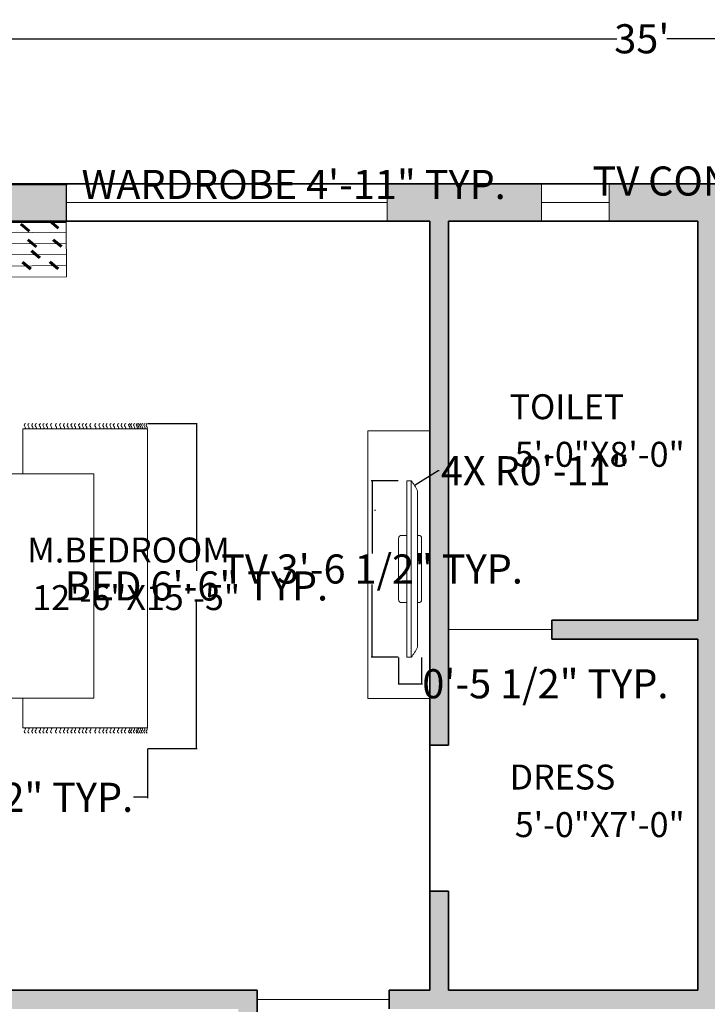
# Model space of a CAD drawing. Units: inches. Extents: x 136 to 672, y -412 to 279.
# Tile 5 of 6: x 244 to 409, y 42 to 279. Entities that reach past the tile are written whole.
import ezdxf

# ---------------------------------------------------------------- set-up
doc = ezdxf.new("R2010")
doc.units = ezdxf.units.IN
doc.header["$MEASUREMENT"] = 0
for name, color, linetype, lineweight in [('A-ANNO-DIMS', 12, 'Continuous', 18), ('A-AREA-IDEN', 7, 'Continuous', 18), ('A-DOOR', 4, 'Continuous', 18), ('A-EQPM', 8, 'Continuous', 18), ('A-FLOR-CASE', 252, 'Continuous', 18), ('A-FLOR-CASE-PATT', 9, 'Continuous', 9), ('A-WALL-PATT', 244, 'Continuous', 9), ('furniture', 252, 'Continuous', 18), ('walls', 253, 'Continuous', 35), ('windows', 171, 'Continuous', 18)]:
    doc.layers.add(name, color=color, linetype=linetype, lineweight=lineweight)
doc.styles.get("Standard").update_dxf_attribs({"font": 'arial.ttf'})
doc.dimstyles.get("Standard").update_dxf_attribs({"dimtxt": 7, "dimasz": 0.18, "dimexe": 0.18, "dimexo": 0.0625, "dimgap": 0.09, "dimtad": 0, "dimtih": 1, "dimtoh": 1, "dimzin": 0, "dimdsep": 46, "dimlunit": 3, "dimtxsty": 'Standard', "dimcen": 0.09, "dimadec": 0, "dimazin": 0, "dimtfac": 1, "dimtofl": 0, "dimtmove": 0, "dimatfit": 3, "dimfxl": 1, "dimtolj": 1, "dimtzin": 0, "dimarcsym": 0})

# ---------------------------------------------------------------- blocks, each defined once
blk = doc.blocks.new('CARPET')
at = {"layer": 'furniture'}
for p, q in [((-51.53, -98.11), (-51.53, -55.12)), ((-51.53, -55.12), (-41.27, -55.12)), ((36, -55.12), (51.55, -55.12)), ((51.55, -55.12), (51.55, -98.11)), ((51.55, -98.11), (-51.53, -98.11))]:
    blk.add_line(p, q, dxfattribs=at)
for points, knots in [([(-53.37, -55.99), (-53.22, -55.8), (-52.9, -55.41), (-52.34, -55.8), (-51.89, -56.08), (-51.65, -55.91), (-51.53, -55.83)], [0, 0, 0, 0, 0.653278, 1.290138, 1.740457, 2.114451, 2.114451, 2.114451, 2.114451]), ([(-53.37, -57.26), (-53.22, -57.07), (-52.9, -56.67), (-52.34, -57.07), (-51.89, -57.35), (-51.65, -57.17), (-51.53, -57.1)], [0, 0, 0, 0, 0.653278, 1.290138, 1.740457, 2.114451, 2.114451, 2.114451, 2.114451]), ([(53.37, -55.99), (53.22, -55.8), (52.9, -55.41), (52.34, -55.8), (51.89, -56.08), (51.65, -55.91), (51.53, -55.83)], [0, 0, 0, 0, 0.653278, 1.290138, 1.740457, 2.114451, 2.114451, 2.114451, 2.114451]), ([(53.37, -57.26), (53.22, -57.07), (52.9, -56.67), (52.34, -57.07), (51.89, -57.35), (51.65, -57.17), (51.53, -57.1)], [0, 0, 0, 0, 0.653278, 1.290138, 1.740457, 2.114451, 2.114451, 2.114451, 2.114451]), ([(-53.37, -58.59), (-53.22, -58.4), (-52.9, -58.01), (-52.34, -58.4), (-51.89, -58.68), (-51.65, -58.5), (-51.53, -58.43)], [0, 0, 0, 0, 0.653278, 1.290138, 1.740457, 2.114451, 2.114451, 2.114451, 2.114451]), ([(-53.37, -59.78), (-53.22, -59.58), (-52.9, -59.19), (-52.34, -59.58), (-51.89, -59.86), (-51.65, -59.69), (-51.53, -59.61)], [0, 0, 0, 0, 0.653278, 1.290138, 1.740457, 2.114451, 2.114451, 2.114451, 2.114451]), ([(-53.37, -61.22), (-53.22, -61.02), (-52.9, -60.63), (-52.34, -61.02), (-51.89, -61.3), (-51.65, -61.13), (-51.53, -61.05)], [0, 0, 0, 0, 0.653278, 1.290138, 1.740457, 2.114451, 2.114451, 2.114451, 2.114451]), ([(53.37, -58.59), (53.22, -58.4), (52.9, -58.01), (52.34, -58.4), (51.89, -58.68), (51.65, -58.5), (51.53, -58.43)], [0, 0, 0, 0, 0.653278, 1.290138, 1.740457, 2.114451, 2.114451, 2.114451, 2.114451]), ([(53.37, -59.78), (53.22, -59.58), (52.9, -59.19), (52.34, -59.58), (51.89, -59.86), (51.65, -59.69), (51.53, -59.61)], [0, 0, 0, 0, 0.653278, 1.290138, 1.740457, 2.114451, 2.114451, 2.114451, 2.114451]), ([(53.37, -61.22), (53.22, -61.02), (52.9, -60.63), (52.34, -61.02), (51.89, -61.3), (51.65, -61.13), (51.53, -61.05)], [0, 0, 0, 0, 0.653278, 1.290138, 1.740457, 2.114451, 2.114451, 2.114451, 2.114451]), ([(-53.37, -62.44), (-53.22, -62.25), (-52.9, -61.86), (-52.34, -62.25), (-51.89, -62.53), (-51.65, -62.36), (-51.53, -62.28)], [0, 0, 0, 0, 0.653278, 1.290138, 1.740457, 2.114451, 2.114451, 2.114451, 2.114451]), ([(-53.37, -63.63), (-53.22, -63.43), (-52.9, -63.04), (-52.34, -63.43), (-51.89, -63.72), (-51.65, -63.54), (-51.53, -63.46)], [0, 0, 0, 0, 0.653278, 1.290138, 1.740457, 2.114451, 2.114451, 2.114451, 2.114451]), ([(53.37, -62.44), (53.22, -62.25), (52.9, -61.86), (52.34, -62.25), (51.89, -62.53), (51.65, -62.36), (51.53, -62.28)], [0, 0, 0, 0, 0.653278, 1.290138, 1.740457, 2.114451, 2.114451, 2.114451, 2.114451]), ([(53.37, -63.63), (53.22, -63.43), (52.9, -63.04), (52.34, -63.43), (51.89, -63.72), (51.65, -63.54), (51.53, -63.46)], [0, 0, 0, 0, 0.653278, 1.290138, 1.740457, 2.114451, 2.114451, 2.114451, 2.114451]), ([(-53.37, -65.07), (-53.22, -64.87), (-52.9, -64.48), (-52.34, -64.87), (-51.89, -65.15), (-51.65, -64.98), (-51.53, -64.9)], [0, 0, 0, 0, 0.653278, 1.290138, 1.740457, 2.114451, 2.114451, 2.114451, 2.114451]), ([(-53.37, -66.76), (-53.22, -66.56), (-52.9, -66.17), (-52.34, -66.56), (-51.89, -66.84), (-51.65, -66.67), (-51.53, -66.59)], [0, 0, 0, 0, 0.653278, 1.290138, 1.740457, 2.114451, 2.114451, 2.114451, 2.114451]), ([(-53.37, -68.2), (-53.22, -68), (-52.9, -67.61), (-52.34, -68), (-51.89, -68.28), (-51.65, -68.11), (-51.53, -68.03)], [0, 0, 0, 0, 0.653278, 1.290138, 1.740457, 2.114451, 2.114451, 2.114451, 2.114451]), ([(53.37, -65.07), (53.22, -64.87), (52.9, -64.48), (52.34, -64.87), (51.89, -65.15), (51.65, -64.98), (51.53, -64.9)], [0, 0, 0, 0, 0.653278, 1.290138, 1.740457, 2.114451, 2.114451, 2.114451, 2.114451]), ([(53.37, -66.76), (53.22, -66.56), (52.9, -66.17), (52.34, -66.56), (51.89, -66.84), (51.65, -66.67), (51.53, -66.59)], [0, 0, 0, 0, 0.653278, 1.290138, 1.740457, 2.114451, 2.114451, 2.114451, 2.114451]), ([(53.37, -68.2), (53.22, -68), (52.9, -67.61), (52.34, -68), (51.89, -68.28), (51.65, -68.11), (51.53, -68.03)], [0, 0, 0, 0, 0.653278, 1.290138, 1.740457, 2.114451, 2.114451, 2.114451, 2.114451]), ([(-53.37, -69.53), (-53.22, -69.33), (-52.9, -68.94), (-52.34, -69.33), (-51.89, -69.61), (-51.65, -69.44), (-51.53, -69.36)], [0, 0, 0, 0, 0.653278, 1.290138, 1.740457, 2.114451, 2.114451, 2.114451, 2.114451]), ([(-53.37, -70.79), (-53.22, -70.6), (-52.9, -70.21), (-52.34, -70.6), (-51.89, -70.88), (-51.65, -70.7), (-51.53, -70.63)], [0, 0, 0, 0, 0.653278, 1.290138, 1.740457, 2.114451, 2.114451, 2.114451, 2.114451]), ([(53.37, -69.53), (53.22, -69.33), (52.9, -68.94), (52.34, -69.33), (51.89, -69.61), (51.65, -69.44), (51.53, -69.36)], [0, 0, 0, 0, 0.653278, 1.290138, 1.740457, 2.114451, 2.114451, 2.114451, 2.114451]), ([(53.37, -70.79), (53.22, -70.6), (52.9, -70.21), (52.34, -70.6), (51.89, -70.88), (51.65, -70.7), (51.53, -70.63)], [0, 0, 0, 0, 0.653278, 1.290138, 1.740457, 2.114451, 2.114451, 2.114451, 2.114451]), ([(-53.37, -72.12), (-53.22, -71.93), (-52.9, -71.54), (-52.34, -71.93), (-51.89, -72.21), (-51.65, -72.04), (-51.53, -71.96)], [0, 0, 0, 0, 0.653278, 1.290138, 1.740457, 2.114451, 2.114451, 2.114451, 2.114451]), ([(-53.37, -73.31), (-53.22, -73.11), (-52.9, -72.72), (-52.34, -73.11), (-51.89, -73.4), (-51.65, -73.22), (-51.53, -73.14)], [0, 0, 0, 0, 0.653278, 1.290138, 1.740457, 2.114451, 2.114451, 2.114451, 2.114451]), ([(-53.37, -74.75), (-53.22, -74.55), (-52.9, -74.16), (-52.34, -74.55), (-51.89, -74.83), (-51.65, -74.66), (-51.53, -74.58)], [0, 0, 0, 0, 0.653278, 1.290138, 1.740457, 2.114451, 2.114451, 2.114451, 2.114451]), ([(53.37, -72.12), (53.22, -71.93), (52.9, -71.54), (52.34, -71.93), (51.89, -72.21), (51.65, -72.04), (51.53, -71.96)], [0, 0, 0, 0, 0.653278, 1.290138, 1.740457, 2.114451, 2.114451, 2.114451, 2.114451]), ([(53.37, -73.31), (53.22, -73.11), (52.9, -72.72), (52.34, -73.11), (51.89, -73.4), (51.65, -73.22), (51.53, -73.14)], [0, 0, 0, 0, 0.653278, 1.290138, 1.740457, 2.114451, 2.114451, 2.114451, 2.114451]), ([(53.37, -74.75), (53.22, -74.55), (52.9, -74.16), (52.34, -74.55), (51.89, -74.83), (51.65, -74.66), (51.53, -74.58)], [0, 0, 0, 0, 0.653278, 1.290138, 1.740457, 2.114451, 2.114451, 2.114451, 2.114451]), ([(-53.37, -75.98), (-53.22, -75.78), (-52.9, -75.39), (-52.34, -75.78), (-51.89, -76.06), (-51.65, -75.89), (-51.53, -75.81)], [0, 0, 0, 0, 0.653278, 1.290138, 1.740457, 2.114451, 2.114451, 2.114451, 2.114451]), ([(-53.37, -77.16), (-53.22, -76.96), (-52.9, -76.57), (-52.34, -76.96), (-51.89, -77.25), (-51.65, -77.07), (-51.53, -76.99)], [0, 0, 0, 0, 0.653278, 1.290138, 1.740457, 2.114451, 2.114451, 2.114451, 2.114451]), ([(53.37, -75.98), (53.22, -75.78), (52.9, -75.39), (52.34, -75.78), (51.89, -76.06), (51.65, -75.89), (51.53, -75.81)], [0, 0, 0, 0, 0.653278, 1.290138, 1.740457, 2.114451, 2.114451, 2.114451, 2.114451]), ([(53.37, -77.16), (53.22, -76.96), (52.9, -76.57), (52.34, -76.96), (51.89, -77.25), (51.65, -77.07), (51.53, -76.99)], [0, 0, 0, 0, 0.653278, 1.290138, 1.740457, 2.114451, 2.114451, 2.114451, 2.114451]), ([(-53.37, -78.6), (-53.22, -78.4), (-52.9, -78.01), (-52.34, -78.4), (-51.89, -78.68), (-51.65, -78.51), (-51.53, -78.43)], [0, 0, 0, 0, 0.653278, 1.290138, 1.740457, 2.114451, 2.114451, 2.114451, 2.114451]), ([(-53.37, -80.29), (-53.22, -80.09), (-52.9, -79.7), (-52.34, -80.09), (-51.89, -80.37), (-51.65, -80.2), (-51.53, -80.12)], [0, 0, 0, 0, 0.653278, 1.290138, 1.740457, 2.114451, 2.114451, 2.114451, 2.114451]), ([(-53.37, -81.73), (-53.22, -81.53), (-52.9, -81.14), (-52.34, -81.53), (-51.89, -81.81), (-51.65, -81.64), (-51.53, -81.56)], [0, 0, 0, 0, 0.653278, 1.290138, 1.740457, 2.114451, 2.114451, 2.114451, 2.114451]), ([(53.37, -78.6), (53.22, -78.4), (52.9, -78.01), (52.34, -78.4), (51.89, -78.68), (51.65, -78.51), (51.53, -78.43)], [0, 0, 0, 0, 0.653278, 1.290138, 1.740457, 2.114451, 2.114451, 2.114451, 2.114451]), ([(53.37, -80.29), (53.22, -80.09), (52.9, -79.7), (52.34, -80.09), (51.89, -80.37), (51.65, -80.2), (51.53, -80.12)], [0, 0, 0, 0, 0.653278, 1.290138, 1.740457, 2.114451, 2.114451, 2.114451, 2.114451]), ([(53.37, -81.73), (53.22, -81.53), (52.9, -81.14), (52.34, -81.53), (51.89, -81.81), (51.65, -81.64), (51.53, -81.56)], [0, 0, 0, 0, 0.653278, 1.290138, 1.740457, 2.114451, 2.114451, 2.114451, 2.114451]), ([(-53.37, -83.06), (-53.22, -82.86), (-52.9, -82.47), (-52.34, -82.86), (-51.89, -83.14), (-51.65, -82.97), (-51.53, -82.89)], [0, 0, 0, 0, 0.653278, 1.290138, 1.740457, 2.114451, 2.114451, 2.114451, 2.114451]), ([(-53.37, -84.18), (-53.22, -83.99), (-52.9, -83.6), (-52.34, -83.99), (-51.89, -84.27), (-51.65, -84.09), (-51.53, -84.02)], [0, 0, 0, 0, 0.653278, 1.290138, 1.740457, 2.114451, 2.114451, 2.114451, 2.114451]), ([(53.37, -83.06), (53.22, -82.86), (52.9, -82.47), (52.34, -82.86), (51.89, -83.14), (51.65, -82.97), (51.53, -82.89)], [0, 0, 0, 0, 0.653278, 1.290138, 1.740457, 2.114451, 2.114451, 2.114451, 2.114451]), ([(53.37, -84.18), (53.22, -83.99), (52.9, -83.6), (52.34, -83.99), (51.89, -84.27), (51.65, -84.09), (51.53, -84.02)], [0, 0, 0, 0, 0.653278, 1.290138, 1.740457, 2.114451, 2.114451, 2.114451, 2.114451]), ([(-53.37, -85.51), (-53.22, -85.32), (-52.9, -84.93), (-52.34, -85.32), (-51.89, -85.6), (-51.65, -85.42), (-51.53, -85.35)], [0, 0, 0, 0, 0.653278, 1.290138, 1.740457, 2.114451, 2.114451, 2.114451, 2.114451]), ([(-53.37, -86.7), (-53.22, -86.5), (-52.9, -86.11), (-52.34, -86.5), (-51.89, -86.78), (-51.65, -86.61), (-51.53, -86.53)], [0, 0, 0, 0, 0.653278, 1.290138, 1.740457, 2.114451, 2.114451, 2.114451, 2.114451]), ([(-53.37, -88.14), (-53.22, -87.94), (-52.9, -87.55), (-52.34, -87.94), (-51.89, -88.22), (-51.65, -88.05), (-51.53, -87.97)], [0, 0, 0, 0, 0.653278, 1.290138, 1.740457, 2.114451, 2.114451, 2.114451, 2.114451]), ([(53.37, -85.51), (53.22, -85.32), (52.9, -84.93), (52.34, -85.32), (51.89, -85.6), (51.65, -85.42), (51.53, -85.35)], [0, 0, 0, 0, 0.653278, 1.290138, 1.740457, 2.114451, 2.114451, 2.114451, 2.114451]), ([(53.37, -86.7), (53.22, -86.5), (52.9, -86.11), (52.34, -86.5), (51.89, -86.78), (51.65, -86.61), (51.53, -86.53)], [0, 0, 0, 0, 0.653278, 1.290138, 1.740457, 2.114451, 2.114451, 2.114451, 2.114451]), ([(53.37, -88.14), (53.22, -87.94), (52.9, -87.55), (52.34, -87.94), (51.89, -88.22), (51.65, -88.05), (51.53, -87.97)], [0, 0, 0, 0, 0.653278, 1.290138, 1.740457, 2.114451, 2.114451, 2.114451, 2.114451]), ([(-53.37, -89.36), (-53.22, -89.17), (-52.9, -88.78), (-52.34, -89.17), (-51.89, -89.45), (-51.65, -89.28), (-51.53, -89.2)], [0, 0, 0, 0, 0.653278, 1.290138, 1.740457, 2.114451, 2.114451, 2.114451, 2.114451]), ([(-53.37, -90.55), (-53.22, -90.35), (-52.9, -89.96), (-52.34, -90.35), (-51.89, -90.64), (-51.65, -90.46), (-51.53, -90.38)], [0, 0, 0, 0, 0.653278, 1.290138, 1.740457, 2.114451, 2.114451, 2.114451, 2.114451]), ([(-53.37, -91.99), (-53.22, -91.79), (-52.9, -91.4), (-52.34, -91.79), (-51.89, -92.07), (-51.65, -91.9), (-51.53, -91.82)], [0, 0, 0, 0, 0.653278, 1.290138, 1.740457, 2.114451, 2.114451, 2.114451, 2.114451]), ([(53.37, -89.36), (53.22, -89.17), (52.9, -88.78), (52.34, -89.17), (51.89, -89.45), (51.65, -89.28), (51.53, -89.2)], [0, 0, 0, 0, 0.653278, 1.290138, 1.740457, 2.114451, 2.114451, 2.114451, 2.114451]), ([(53.37, -90.55), (53.22, -90.35), (52.9, -89.96), (52.34, -90.35), (51.9, -90.63), (51.66, -90.47), (51.55, -90.4)], [0, 0, 0, 0, 0.653278, 1.290138, 1.740457, 2.0926, 2.0926, 2.0926, 2.0926]), ([(53.37, -91.99), (53.22, -91.79), (52.9, -91.4), (52.34, -91.79), (51.9, -92.07), (51.66, -91.91), (51.55, -91.83)], [0, 0, 0, 0, 0.653278, 1.290138, 1.740457, 2.0926, 2.0926, 2.0926, 2.0926]), ([(-53.37, -92.69), (-53.22, -92.48), (-52.9, -92.08), (-52.35, -92.49), (-51.89, -92.77), (-51.65, -92.6), (-51.53, -92.52)], [0, 0, 0, 0, 0.663904, 1.307406, 1.757725, 2.131719, 2.131719, 2.131719, 2.131719]), ([(-53.37, -93.61), (-53.22, -93.42), (-52.9, -93.03), (-52.34, -93.42), (-51.89, -93.7), (-51.65, -93.52), (-51.53, -93.45)], [0, 0, 0, 0, 0.653278, 1.290138, 1.740457, 2.114451, 2.114451, 2.114451, 2.114451]), ([(-53.37, -94.55), (-53.22, -94.35), (-52.9, -93.96), (-52.34, -94.35), (-51.89, -94.63), (-51.65, -94.46), (-51.53, -94.38)], [0, 0, 0, 0, 0.653278, 1.290138, 1.740457, 2.114451, 2.114451, 2.114451, 2.114451]), ([(-53.37, -95.05), (-53.22, -94.85), (-52.9, -94.46), (-52.34, -94.85), (-51.89, -95.14), (-51.65, -94.96), (-51.53, -94.88)], [0, 0, 0, 0, 0.653278, 1.290138, 1.740457, 2.114451, 2.114451, 2.114451, 2.114451]), ([(53.37, -92.69), (53.22, -92.49), (52.9, -92.09), (52.34, -92.49), (51.9, -92.77), (51.66, -92.61), (51.55, -92.53)], [0, 0, 0, 0, 0.656792, 1.295826, 1.746145, 2.098292, 2.098292, 2.098292, 2.098292]), ([(53.37, -93.66), (53.22, -93.46), (52.9, -93.07), (52.34, -93.46), (51.9, -93.74), (51.66, -93.58), (51.55, -93.5)], [0, 0, 0, 0, 0.653278, 1.290138, 1.740457, 2.0926, 2.0926, 2.0926, 2.0926]), ([(53.37, -94.59), (53.22, -94.4), (52.9, -94.01), (52.34, -94.4), (51.9, -94.68), (51.66, -94.51), (51.55, -94.44)], [0, 0, 0, 0, 0.653278, 1.290138, 1.740457, 2.0926, 2.0926, 2.0926, 2.0926]), ([(53.37, -95.1), (53.22, -94.9), (52.9, -94.51), (52.34, -94.9), (51.9, -95.18), (51.66, -95.02), (51.55, -94.94)], [0, 0, 0, 0, 0.653278, 1.290138, 1.740457, 2.0926, 2.0926, 2.0926, 2.0926]), ([(-53.37, -95.73), (-53.22, -95.54), (-52.9, -95.15), (-52.34, -95.54), (-51.89, -95.82), (-51.65, -95.65), (-51.53, -95.57)], [0, 0, 0, 0, 0.653278, 1.290138, 1.740457, 2.114451, 2.114451, 2.114451, 2.114451]), ([(-53.37, -96.38), (-53.22, -96.18), (-52.9, -95.79), (-52.34, -96.18), (-51.89, -96.47), (-51.65, -96.29), (-51.53, -96.21)], [0, 0, 0, 0, 0.653278, 1.290138, 1.740457, 2.114451, 2.114451, 2.114451, 2.114451]), ([(-53.37, -97.17), (-53.22, -96.98), (-52.9, -96.59), (-52.34, -96.98), (-51.89, -97.26), (-51.65, -97.08), (-51.53, -97.01)], [0, 0, 0, 0, 0.653278, 1.290138, 1.740457, 2.114451, 2.114451, 2.114451, 2.114451]), ([(-53.37, -97.99), (-53.22, -97.79), (-52.9, -97.4), (-52.34, -97.79), (-51.89, -98.08), (-51.65, -97.9), (-51.53, -97.82)], [0, 0, 0, 0, 0.653278, 1.290138, 1.740457, 2.114451, 2.114451, 2.114451, 2.114451]), ([(53.37, -95.78), (53.22, -95.58), (52.9, -95.19), (52.34, -95.58), (51.89, -95.86), (51.65, -95.69), (51.53, -95.61)], [0, 0, 0, 0, 0.653278, 1.290138, 1.740457, 2.114451, 2.114451, 2.114451, 2.114451]), ([(53.37, -96.43), (53.22, -96.23), (52.9, -95.84), (52.34, -96.23), (51.89, -96.51), (51.65, -96.34), (51.53, -96.26)], [0, 0, 0, 0, 0.653278, 1.290138, 1.740457, 2.114451, 2.114451, 2.114451, 2.114451]), ([(53.37, -97.22), (53.22, -97.02), (52.9, -96.63), (52.34, -97.02), (51.89, -97.3), (51.65, -97.13), (51.53, -97.05)], [0, 0, 0, 0, 0.653278, 1.290138, 1.740457, 2.114451, 2.114451, 2.114451, 2.114451]), ([(53.37, -97.99), (53.22, -97.79), (52.9, -97.4), (52.34, -97.79), (51.89, -98.08), (51.65, -97.9), (51.53, -97.82)], [0, 0, 0, 0, 0.653278, 1.290138, 1.740457, 2.114451, 2.114451, 2.114451, 2.114451])]:
    blk.add_open_spline(points, degree=3, knots=knots, dxfattribs=at)
blk = doc.blocks.new('A$C58D270C6')
at = {"layer": 'furniture'}
for p, q in [((9.09, 124.13), (9.09, 108.87)), ((1.46, 116.5), (16.73, 116.5)), ((14.97, 94.84), (24.62, 107.92)), ((24.62, 94.93), (24.62, 107.92)), ((42.08, 108), (42.08, 36)), ((14.97, 94.93), (24.62, 94.93)), ((14.97, 94.84), (14.97, 36)), ((16.22, 94.93), (16.22, 36)), ((9.25, 36), (9.25, 20.74)), ((1.62, 28.37), (16.88, 28.37))]:
    blk.add_line(p, q, dxfattribs=at)
for points in [[(18.5, 108), (18.34, 124.13), (-0.16, 124.13), (0, 108)], [(0, 108), (77.91, 108), (77.91, 36), (0, 36)], [(4.09, 94.93), (14.97, 94.93), (14.97, 73.83), (4.09, 73.83)], [(4.09, 65.23), (14.97, 65.23), (14.97, 44.13), (4.09, 44.13)], [(18.65, 19.87), (18.5, 36), (0, 36), (0.16, 19.87)]]:
    blk.add_lwpolyline(points, close=True, dxfattribs=at)
for centre in [(9.09, 116.5), (9.25, 28.37)]:
    blk.add_circle(centre, 5.95, dxfattribs=at)
at = {"layer": 'furniture', "xscale": 0.9312884925094044, "yscale": 0.9312884925094044, "zscale": 0.9312884925094044, "rotation": 90}
blk.add_blockref('CARPET', (3.79, 74.47), dxfattribs=at)
blk = doc.blocks.new('PLASMA-LARGE')
at = {"layer": 'furniture'}
for p, q in [((-7.26, 0), (7.26, 0)), ((-18.61, -1), (18.61, -1)), ((-8, -1), (-8, -0.74)), ((8, -1), (8, -0.74)), ((-21, -2.5), (21, -2.5)), ((-21, -2.5), (-21, -3.5)), ((-21, -3.5), (21, -3.5)), ((-8, -3.5), (-8, -4.76)), ((8, -3.5), (8, -4.76)), ((21, -2.5), (21, -3.5)), ((-7.26, -5.5), (7.26, -5.5))]:
    blk.add_line(p, q, dxfattribs=at)
for centre, radius, start, end in [((-7.26, -0.74), 0.744, 90, 180), ((7.26, -0.74), 0.744, 0, 90), ((-13.97, -11.05), 11.07, 114.7602, 129.4175), ((13.97, -11.05), 11.07, 50.5825, 65.2398), ((-7.26, -4.76), 0.744, 180, 270), ((7.26, -4.76), 0.744, 270, 0)]:
    blk.add_arc(centre, radius, start, end, dxfattribs=at)
blk = doc.blocks.new('*D18')
at = {"layer": 'A-ANNO-DIMS', "color": 0, "lineweight": -2, "transparency": 16777216}
for p, q in [((183.46, 273.1), (183.46, 274.63)), ((183.64, 274.45), (387.44, 274.45)), ((603.28, 274.45), (399.49, 274.45)), ((603.46, 273.1), (603.46, 274.63))]:
    blk.add_line(p, q, dxfattribs=at)
at = {"layer": 'A-ANNO-DIMS', "color": 0, "transparency": 16777216}
for points in [[(183.64, 274.48), (183.64, 274.42), (183.46, 274.45)], [(603.28, 274.48), (603.28, 274.42), (603.46, 274.45)]]:
    blk.add_solid(points, dxfattribs=at)
at = {"layer": 'Defpoints', "color": 0, "transparency": 16777216}
for p in [(183.46, 273.04), (603.46, 274.45), (603.46, 273.04)]:
    blk.add_point(p, dxfattribs=at)
at = {"layer": 'A-ANNO-DIMS', "color": 0, "transparency": 16777216, "insert": (393.46, 274.45), "char_height": 7, "attachment_point": 5}
blk.add_mtext("\\A1;35'", dxfattribs=at)
blk = doc.blocks.new('WIN-16')
for p, q in [((0, 16.27), (9, 16.27)), ((0, 0), (0, 16.27)), ((0, 16.27), (4.5, 16.27)), ((4.5, 16.27), (4.5, 0)), ((9, 16.27), (9, 0)), ((9, 0), (0, 0))]:
    blk.add_line(p, q)
blk = doc.blocks.new('CONSOLE-TV')
for p, q in [((0, 0), (0, 64.44)), ((0, 64.44), (14.9, 64.44)), ((14.9, 0), (0, 0))]:
    blk.add_line(p, q)
blk = doc.blocks.new('WARDROBE-FRAME')
for p, q in [((0, 13.37), (58.88, 13.37)), ((0.05, 13.37), (0.13, 0)), ((58.95, 0.34), (58.88, 13.71)), ((0.02, 10.69), (58.89, 11.04)), ((0.03, 8.02), (58.91, 8.36)), ((0.05, 5.35), (58.92, 5.69)), ((0.06, 2.67), (58.94, 3.02)), ((0.08, 0), (58.95, 0.34))]:
    blk.add_line(p, q)
blk = doc.blocks.new('*D27')
at = {"layer": 'A-ANNO-DIMS', "color": 0, "lineweight": -2, "transparency": 16777216}
for p, q in [((274.68, 181.94), (286.53, 181.94)), ((286.35, 181.76), (286.35, 146.49)), ((286.35, 103.9), (286.35, 139.16)), ((274.68, 103.72), (286.53, 103.72))]:
    blk.add_line(p, q, dxfattribs=at)
at = {"layer": 'A-ANNO-DIMS', "color": 0, "transparency": 16777216}
for points in [[(286.32, 181.76), (286.38, 181.76), (286.35, 181.94)], [(286.32, 103.9), (286.38, 103.9), (286.35, 103.72)]]:
    blk.add_solid(points, dxfattribs=at)
at = {"layer": 'Defpoints', "color": 0, "transparency": 16777216}
for p in [(274.61, 181.94), (286.35, 181.94), (274.61, 103.72)]:
    blk.add_point(p, dxfattribs=at)
at = {"layer": 'A-ANNO-DIMS', "color": 0, "transparency": 16777216, "insert": (286.35, 142.83), "char_height": 7, "attachment_point": 5}
blk.add_mtext('\\A1;BED 6\'-6" TYP.', dxfattribs=at)
blk = doc.blocks.new('*D28')
at = {"layer": 'A-ANNO-DIMS', "color": 0, "lineweight": -2, "transparency": 16777216}
for p, q in [((203.15, 103.66), (203.15, 91.81)), ((274.61, 103.66), (274.61, 91.81)), ((203.33, 91.99), (206.58, 91.99)), ((274.43, 91.99), (271.18, 91.99))]:
    blk.add_line(p, q, dxfattribs=at)
at = {"layer": 'A-ANNO-DIMS', "color": 0, "transparency": 16777216}
for points in [[(203.33, 92.02), (203.33, 91.96), (203.15, 91.99)], [(274.43, 92.02), (274.43, 91.96), (274.61, 91.99)]]:
    blk.add_solid(points, dxfattribs=at)
at = {"layer": 'Defpoints', "color": 0, "transparency": 16777216}
for p in [(203.15, 103.72), (274.61, 103.72), (274.61, 91.99)]:
    blk.add_point(p, dxfattribs=at)
at = {"layer": 'A-ANNO-DIMS', "color": 0, "transparency": 16777216, "insert": (238.88, 91.99), "char_height": 7, "attachment_point": 5}
blk.add_mtext('\\A1;5\'-11 1/2" TYP.', dxfattribs=at)
blk = doc.blocks.new('*D29')
at = {"layer": 'A-ANNO-DIMS', "color": 0, "lineweight": -2, "transparency": 16777216}
for p, q in [((196.15, 230.63), (196.15, 239.59)), ((196.33, 239.41), (254.92, 239.41)), ((255.1, 230.63), (255.1, 239.59)), ((255.1, 239.41), (255.28, 239.41))]:
    blk.add_line(p, q, dxfattribs=at)
at = {"layer": 'A-ANNO-DIMS', "color": 0, "transparency": 16777216}
for points in [[(196.33, 239.44), (196.33, 239.38), (196.15, 239.41)], [(254.92, 239.44), (254.92, 239.38), (255.1, 239.41)]]:
    blk.add_solid(points, dxfattribs=at)
at = {"layer": 'Defpoints', "color": 0, "transparency": 16777216}
for p in [(255.1, 239.41), (196.15, 230.56), (255.1, 230.56)]:
    blk.add_point(p, dxfattribs=at)
at = {"layer": 'A-ANNO-DIMS', "color": 0, "transparency": 16777216, "insert": (309.72, 239.41), "char_height": 7, "attachment_point": 5}
blk.add_mtext('\\A1;WARDROBE 4\'-11" TYP.', dxfattribs=at)
blk = doc.blocks.new('*D31')
at = {"layer": 'A-ANNO-DIMS', "color": 0, "lineweight": -2, "transparency": 16777216}
for p, q in [((503.53, 240.23), (503.35, 240.23)), ((503.53, 230.63), (503.53, 240.41)), ((567.79, 240.23), (503.71, 240.23)), ((567.97, 230.63), (567.97, 240.41))]:
    blk.add_line(p, q, dxfattribs=at)
at = {"layer": 'A-ANNO-DIMS', "color": 0, "transparency": 16777216}
for points in [[(503.71, 240.26), (503.71, 240.2), (503.53, 240.23)], [(567.79, 240.26), (567.79, 240.2), (567.97, 240.23)]]:
    blk.add_solid(points, dxfattribs=at)
at = {"layer": 'Defpoints', "color": 0, "transparency": 16777216}
for p in [(503.53, 240.23), (503.53, 230.56), (567.97, 230.56)]:
    blk.add_point(p, dxfattribs=at)
at = {"layer": 'A-ANNO-DIMS', "color": 0, "transparency": 16777216, "insert": (440.81, 240.23), "char_height": 7, "attachment_point": 5}
blk.add_mtext('\\A1;TV CONSOLE 5\'-4 1/2" TYP.', dxfattribs=at)
blk = doc.blocks.new('*D33')
at = {"layer": 'A-ANNO-DIMS', "color": 0, "lineweight": -2, "transparency": 16777216}
for p, q in [((334.89, 168.15), (328.4, 168.15)), ((328.58, 167.97), (328.58, 150.62)), ((328.58, 125.85), (328.58, 143.2)), ((334.89, 125.67), (328.4, 125.67))]:
    blk.add_line(p, q, dxfattribs=at)
at = {"layer": 'A-ANNO-DIMS', "color": 0, "transparency": 16777216}
for points in [[(328.55, 167.97), (328.61, 167.97), (328.58, 168.15)], [(328.55, 125.85), (328.61, 125.85), (328.58, 125.67)]]:
    blk.add_solid(points, dxfattribs=at)
at = {"layer": 'Defpoints', "color": 0, "transparency": 16777216}
for p in [(334.95, 168.15), (328.58, 125.67), (334.95, 125.67)]:
    blk.add_point(p, dxfattribs=at)
at = {"layer": 'A-ANNO-DIMS', "color": 0, "transparency": 16777216, "insert": (328.58, 146.91), "char_height": 7, "attachment_point": 5}
blk.add_mtext('\\A1;TV 3\'-6 1/2" TYP.', dxfattribs=at)
blk = doc.blocks.new('*D34')
at = {"layer": 'A-ANNO-DIMS', "color": 0, "lineweight": -2, "transparency": 16777216}
for p, q in [((334.95, 125.61), (334.95, 119.12)), ((340.51, 125.61), (340.51, 119.12)), ((335.13, 119.3), (340.33, 119.3)), ((340.51, 119.3), (340.69, 119.3))]:
    blk.add_line(p, q, dxfattribs=at)
at = {"layer": 'A-ANNO-DIMS', "color": 0, "transparency": 16777216}
for points in [[(335.13, 119.33), (335.13, 119.27), (334.95, 119.3)], [(340.33, 119.33), (340.33, 119.27), (340.51, 119.3)]]:
    blk.add_solid(points, dxfattribs=at)
at = {"layer": 'Defpoints', "color": 0, "transparency": 16777216}
for p in [(334.95, 125.67), (340.51, 125.67), (340.51, 119.3)]:
    blk.add_point(p, dxfattribs=at)
at = {"layer": 'A-ANNO-DIMS', "color": 0, "transparency": 16777216, "insert": (370.27, 119.3), "char_height": 7, "attachment_point": 5}
blk.add_mtext('\\A1;0\'-5 1/2" TYP.', dxfattribs=at)
blk = doc.blocks.new('*D57')
at = {"layer": 'A-ANNO-DIMS', "color": 0, "lineweight": -2, "transparency": 16777216}
for p, q in [((344.51, 170.55), (338.97, 167.08)), ((344.69, 170.55), (344.51, 170.55)), ((329.34, 160.95), (329.34, 161.13)), ((329.25, 161.04), (329.43, 161.04))]:
    blk.add_line(p, q, dxfattribs=at)
at = {"layer": 'A-ANNO-DIMS', "color": 0, "transparency": 16777216}
blk.add_solid([(338.96, 167.11), (338.99, 167.06), (338.82, 166.99)], dxfattribs=at)
at = {"layer": 'Defpoints', "color": 0, "transparency": 16777216}
for p in [(338.82, 166.99), (329.34, 161.04)]:
    blk.add_point(p, dxfattribs=at)
at = {"layer": 'A-ANNO-DIMS', "color": 0, "transparency": 16777216, "insert": (367.81, 170.55), "char_height": 7, "attachment_point": 5}
blk.add_mtext('\\A1;4X R0\'-11"', dxfattribs=at)

msp = doc.modelspace()

# ---------------------------------------------------------------- hatches: boundary and pattern name
at = {"layer": 'A-FLOR-CASE-PATT'}
h = msp.add_hatch(dxfattribs=at)
h.set_pattern_fill('ANSI31', color=256, scale=0.8475512, angle=95.46701, style=0)
h.paths.add_polyline_path([(246.274, 228.354), (244.277, 230.002), (244.003, 229.67), (246, 228.022)])
h = msp.add_hatch(dxfattribs=at)
h.set_pattern_fill('ANSI31', color=256, scale=0.8476353, angle=95.46701, style=0)
h.paths.add_polyline_path([(253.272, 229.078), (251.275, 230.726), (251.001, 230.395), (252.998, 228.747)])
h = msp.add_hatch(dxfattribs=at)
h.set_pattern_fill('ANSI31', color=256, scale=0.8475015, angle=95.46701, style=0)
h.paths.add_polyline_path([(247.971, 224.593), (245.974, 226.241), (245.7, 225.91), (247.697, 224.262)])
h = msp.add_hatch(dxfattribs=at)
h.set_pattern_fill('ANSI31', color=256, scale=0.8474192, angle=95.46701, style=0)
h.paths.add_polyline_path([(254.035, 224.629), (252.038, 226.277), (251.764, 225.945), (253.761, 224.297)])
h = msp.add_hatch(dxfattribs=at)
h.set_pattern_fill('ANSI31', color=256, scale=0.847418, angle=95.467, style=0)
h.paths.add_polyline_path([(248.823, 221.925), (246.826, 223.573), (246.552, 223.241), (248.549, 221.593)])
h = msp.add_hatch(dxfattribs=at)
h.set_pattern_fill('ANSI31', color=256, scale=0.8475127, angle=95.46701, style=0)
h.paths.add_polyline_path([(246.643, 219.239), (244.646, 220.887), (244.372, 220.555), (246.369, 218.907)])
h = msp.add_hatch(dxfattribs=at)
h.set_pattern_fill('ANSI31', color=256, scale=0.8474735, angle=95.46701, style=0)
h.paths.add_polyline_path([(253.23, 219.278), (251.233, 220.926), (250.959, 220.594), (252.956, 218.946)])
at = {"layer": 'A-WALL-PATT'}
h = msp.add_hatch(color=256, dxfattribs=at)
h.dxf.hatch_style = 1
h.paths.add_polyline_path([(255.026, 239.565), (183.463, 239.565), (183.463, 125.252), (187.963, 125.252), (192.463, 125.252), (192.463, 230.565), (255.024, 230.565), (255.025, 235.065)])
h.paths.add_polyline_path([(369.355, 239.565), (332.259, 239.565), (332.259, 230.565), (342.463, 230.565), (342.463, 104.521), (346.963, 104.521), (346.963, 230.565), (369.355, 230.565), (369.355, 235.065)])
h.paths.add_polyline_path([(603.463, 239.565), (385.627, 239.565), (385.627, 230.565), (406.963, 230.565), (406.963, 134.565), (371.802, 134.565), (371.802, 130.065), (406.963, 130.065), (406.963, 45.565), (346.963, 45.565), (346.963, 69.395), (342.463, 69.395), (342.463, 45.565), (332.733, 45.565), (332.733, 41.065), (416.87, 41.065), (416.87, 45.565), (411.463, 45.565), (411.463, 230.565), (594.463, 230.565), (594.463, 199.893), (598.963, 199.893), (603.463, 199.893)])
h.paths.add_polyline_path([(603.463, 145.845), (594.463, 145.845), (594.463, 98.065), (524.374, 98.065), (512.275, 97.948), (512.275, 98.065), (484.021, 98.065), (484.021, 93.565), (505.963, 93.565), (594.463, 93.565), (594.463, 80.073), (598.963, 80.073), (603.463, 80.073)], flags=17)
h.paths.add_polyline_path([(457.963, 98.065), (453.463, 98.065), (453.463, 41.065), (594.463, 41.065), (594.463, -67.933), (603.463, -67.933), (603.463, 63.801), (594.463, 63.801), (594.463, 45.565), (510.463, 45.565), (510.463, 65.243), (505.963, 65.243), (505.963, 45.565), (457.963, 45.565)])
h.paths.add_polyline_path([(192.463, 71.205), (183.463, 71.205), (183.463, 25.824), (192.463, 25.824), (192.463, 41.065), (296.463, 41.065), (296.463, 24.884), (300.963, 24.884), (300.963, 45.565), (192.463, 45.565)])
h.paths.add_polyline_path([(300.963, -6.935), (296.463, -6.935), (192.463, -6.935), (192.463, -11.435), (300.963, -11.435)])
h.paths.add_polyline_path([(192.463, 8.674), (183.463, 8.674), (183.463, -44.733), (187.963, -44.733), (192.463, -44.733)])
h.paths.add_polyline_path([(235.886, -349.935), (192.463, -349.935), (192.463, -358.935), (235.886, -358.935)])
h.paths.add_polyline_path([(345.463, -316.935), (361.986, -316.935), (361.986, -307.935), (340.963, -307.935), (340.963, -229.935), (356.354, -229.935), (356.354, -225.435), (336.463, -225.435), (336.463, -349.935), (300.655, -349.935), (300.655, -358.935), (345.463, -358.935)])
h.paths.add_polyline_path([(407.452, -307.935), (403.463, -307.935), (403.463, -225.435), (382.286, -225.435), (382.286, -229.935), (398.963, -229.935), (398.963, -307.935), (379.137, -307.935), (379.137, -316.935), (407.452, -316.935)])
h.paths.add_polyline_path([(470.463, -284.28), (461.463, -284.28), (461.463, -307.935), (461.463, -316.935), (470.463, -316.935)])
h.paths.add_polyline_path([(470.463, -234.435), (480.349, -234.435), (480.349, -225.435), (461.463, -225.435), (461.463, -245.135), (470.463, -245.135)])
h.paths.add_polyline_path([(603.463, -121.943), (594.463, -121.943), (594.463, -225.435), (574.368, -225.435), (574.368, -234.435), (603.463, -234.435)])
h.paths.add_polyline_path([(340.963, -75.678), (336.463, -75.678), (336.463, -168.061), (340.963, -168.061)])
h.paths.add_polyline_path([(468.637, 59.14), (510.671, 59.14), (510.671, 68.331), (468.637, 68.331)], flags=25)
h.paths.add_polyline_path([(192.463, -208.04), (183.463, -208.04), (183.463, -360.435), (192.463, -360.435)])
h.paths.add_polyline_path([(183.463, -153.992), (192.463, -153.992), (192.463, -98.781), (183.463, -98.781)])

# ---------------------------------------------------------------- linework, layer by layer
at = {"layer": 'A-DOOR'}
for p, q in [((371.802, 132.315), (346.963, 132.315)), ((332.733, 43.315), (300.963, 43.315))]:
    msp.add_line(p, q, dxfattribs=at)
at = {"layer": 'A-FLOR-CASE'}
msp.add_line((251.16, 230.542), (251.491, 230.544), dxfattribs=at)
at = {"layer": 'walls'}
for p, q in [((183.463, 239.565), (603.463, 239.565)), ((192.463, 230.565), (342.463, 230.565)), ((342.463, 45.565), (342.463, 230.565)), ((346.963, 230.565), (406.963, 230.565)), ((346.963, 104.521), (346.963, 230.565)), ((406.963, 134.565), (406.963, 230.565)), ((371.802, 134.565), (406.963, 134.565)), ((371.802, 134.565), (371.802, 130.065)), ((371.802, 130.065), (406.963, 130.065)), ((406.963, 45.565), (406.963, 130.065)), ((342.463, 104.521), (346.963, 104.521)), ((342.463, 69.395), (346.963, 69.395)), ((346.963, 45.565), (346.963, 69.395)), ((192.463, 45.565), (300.963, 45.565)), ((300.963, 24.884), (300.963, 45.565)), ((332.733, 45.565), (332.733, 41.065)), ((332.733, 45.565), (342.463, 45.565)), ((346.963, 45.565), (406.963, 45.565))]:
    msp.add_line(p, q, dxfattribs=at)
at = {"layer": 'windows'}
for p, q in [((255.024, 230.565), (255.026, 239.565)), ((255.026, 239.565), (332.259, 239.565)), ((332.259, 239.565), (332.259, 230.565)), ((255.024, 230.582), (255.025, 235.065)), ((255.025, 235.065), (332.259, 235.065)), ((332.259, 230.565), (255.024, 230.582))]:
    msp.add_line(p, q, dxfattribs=at)

# ---------------------------------------------------------------- block references
at = {"layer": 'A-EQPM', "xscale": 1.011294184530666, "yscale": 1.011294184530666, "zscale": 1.011294184530666, "rotation": 270}
msp.add_blockref('PLASMA-LARGE', (340.512, 146.909), dxfattribs=at)
at = {"layer": 'A-FLOR-CASE'}
for name, p in [('WARDROBE-FRAME', (196.149, 216.854)), ('CONSOLE-TV', (327.566, 115.728))]:
    msp.add_blockref(name, p, dxfattribs=at)
at = {"layer": 'furniture', "xscale": 0.7498206902034922, "yscale": 0.7498206902034922, "zscale": 0.7498206902034922}
msp.add_blockref('A$C58D270C6', (203.262, 88.822), dxfattribs=at)
at = {"layer": 'windows', "rotation": 90.00000000000031}
msp.add_blockref('WIN-16', (385.627, 230.565), dxfattribs=at)

# ---------------------------------------------------------------- texts
at = {"layer": 'A-AREA-IDEN'}
for s, p in [('TOILET', (361.68, 182.943)), ('5\'-0"X8\'-0"', (362.918, 171.496)), ('M.BEDROOM', (245.649, 148.469)), ('12\'-6"X15\'-5"', (246.886, 137.021)), ('DRESS', (361.68, 93.86)), ('5\'-0"X7\'-0"', (362.918, 82.413))]:
    msp.add_text(s, height=6, dxfattribs=at).set_placement(p)

# ---------------------------------------------------------------- dimensions: what is measured, and where the dimension line sits
at = {"layer": 'A-ANNO-DIMS'}
dim = msp.add_linear_dim(base=(603.463, 274.45), p1=(183.463, 273.039), p2=(603.463, 273.039), dimstyle='Standard', override={"dimclrd": 0, "dimclre": 0, "dimclrt": 0}, dxfattribs=at)
dim.commit()
dim.dimension.update_dxf_attribs({"geometry": '*D18', "text_midpoint": (393.463, 274.45)})
for base, p1, p2, angle, text, picture, middle in [((503.53, 240.231), (567.973, 230.565), (503.53, 230.565), 180, 'TV CONSOLE <> TYP.', '*D31', (440.807, 240.231)), ((286.346, 181.935), (274.614, 103.72), (274.614, 181.935), 90, 'BED <> TYP.', '*D27', (286.346, 142.828)), ((328.579, 125.672), (334.95, 168.147), (334.95, 125.672), 270, 'TV <> TYP.', '*D33', (328.579, 146.909))]:
    dim = msp.add_linear_dim(base=base, p1=p1, p2=p2, angle=angle, text=text, dimstyle='Standard', override={"dimdec": 1, "dimlfac": 1, "dimrnd": 0, "dimzin": 1, "dimdsep": 46, "dimlunit": 4, "dimfrac": 2}, dxfattribs=at)
    dim.commit()
    dim.dimension.update_dxf_attribs({"geometry": picture, "text_midpoint": middle})
for base, p1, p2, text, picture, middle in [((255.103, 239.408), (196.149, 230.565), (255.103, 230.565), 'WARDROBE <> TYP.', '*D29', (309.723, 239.408)), ((340.512, 119.301), (334.95, 125.672), (340.512, 125.672), '<> TYP.', '*D34', (370.272, 119.301)), ((274.614, 91.988), (203.145, 103.72), (274.614, 103.72), '<> TYP.', '*D28', (238.88, 91.988))]:
    dim = msp.add_linear_dim(base=base, p1=p1, p2=p2, text=text, dimstyle='Standard', override={"dimdec": 1, "dimlfac": 1, "dimrnd": 0, "dimzin": 1, "dimdsep": 46, "dimlunit": 4, "dimfrac": 2}, dxfattribs=at)
    dim.commit()
    dim.dimension.update_dxf_attribs({"geometry": picture, "text_midpoint": middle})
dim = msp.add_radius_dim(center=(329.337, 161.04), mpoint=(338.82, 166.986), text='4X <>', dimstyle='Standard', override={"dimdec": 1, "dimlfac": 1, "dimrnd": 0, "dimzin": 1, "dimdsep": 46, "dimlunit": 4, "dimfrac": 2}, dxfattribs=at)
dim.commit()
dim.dimension.update_dxf_attribs({"geometry": '*D57', "text_midpoint": (367.814, 170.554), "dimtype": 164})

doc.saveas('drawing.dxf')
